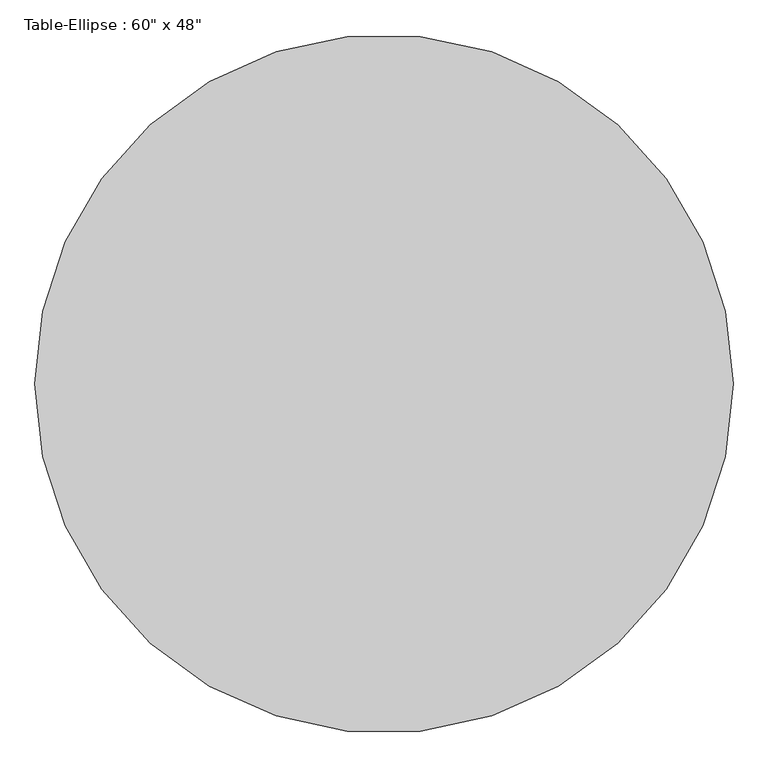
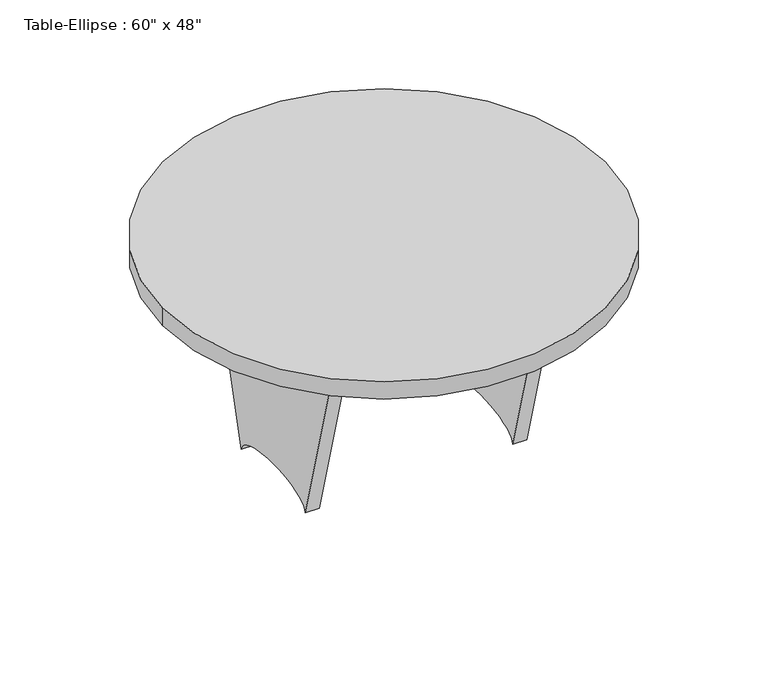
"""IFC4 building model written with IfcOpenShell, lengths in millimetres: furniture geometry."""

from ifc_helpers import new_model, si_unit, point, frame, origin, place, context, project, spatial, circle_curve, ellipse_curve, trimmed, source, transform, mapped, element, save
from ifc_brep_helpers import plane_surface, extruded_surface, advanced_brep


def furniture_c897acec(model_context):
    return source(origin(), model_context, "Body", "AdvancedBrep", [
        advanced_brep(
        [(-266.7, 19.05, 558.8), (266.7, 19.05, 558.8), (266.7, 19.05, 372.5333333), (-266.7, 19.05, 372.5333333), (-266.7, -19.05, 558.8), (-266.7, -19.05, 372.5333333), (266.7, -19.05, 372.5333333), (266.7, -19.05, 558.8)],
        [
            (0, 1),
            (1, 2),
            (2, 3, ellipse_curve(frame((0.0, 19.05, 372.5333333), z_axis=(0.0, -1.0, 0.0), x_axis=(1.0, 0.0, 0.0)), 266.7, 101.6)),
            (3, 0),
            (4, 5),
            (5, 6, ellipse_curve(frame((0.0, -19.05, 372.5333333), z_axis=(0.0, 1.0, 0.0), x_axis=(1.0, 0.0, 0.0)), 266.7, 101.6)),
            (6, 7),
            (7, 4),
            (0, 4),
            (7, 1),
            (6, 2),
            (5, 3),
        ],
        [
            plane_surface(frame((-266.7, 19.05, 558.8), z_axis=(0.0, 1.0, 0.0), x_axis=(1.0, 0.0, 0.0))),
            plane_surface(frame((-266.7, -19.05, 558.8), z_axis=(0.0, -1.0, 0.0), x_axis=(-1.0, 0.0, 0.0))),
            plane_surface(frame((-266.7, 19.05, 558.8), z_axis=(0.0, 0.0, 1.0), x_axis=(0.0, -1.0, 0.0))),
            plane_surface(frame((266.7, 19.05, 558.8), z_axis=(1.0, 0.0, 0.0), x_axis=(0.0, -1.0, 0.0))),
            extruded_surface(trimmed(ellipse_curve(frame((0.0, -57.15, 372.5333333), z_axis=(0.0, -1.0, 0.0), x_axis=(1.0, 0.0, 0.0)), 266.7, 101.6), [point((266.7, -57.15, 372.5333333))], [point((-266.7, -57.15, 372.5333333))], True, "CARTESIAN"), (0.0, 38.099999999999994, 0.0), 38.099999999999994),
            plane_surface(frame((-266.7, 19.05, 372.5333333), z_axis=(-1.0, 0.0, 0.0), x_axis=(0.0, -1.0, 0.0))),
        ],
        [
            (0, [[1, 2, 3, 4]]),
            (1, [[5, 6, 7, 8]]),
            (2, [[-1, 9, -8, 10]]),
            (3, [[-2, -10, -7, 11]]),
            (4, [[-3, -11, -6, 12]]),
            (5, [[-4, -12, -5, -9]]),
        ],
    ),
        advanced_brep(
        [(304.8, 304.8, 558.8), (304.8, -304.8, 558.8), (304.8, -152.4, 0.0), (304.8, 152.4, 0.0), (266.7, 304.8, 558.8), (266.7, 152.4, 0.0), (266.7, -152.4, 0.0), (266.7, -304.8, 558.8)],
        [
            (0, 1),
            (1, 2),
            (2, 3, ellipse_curve(frame((304.8, 0.0, 0.0), z_axis=(-1.0, 0.0, 0.0), x_axis=(0.0, 1.0, 0.0)), 152.4, 50.8)),
            (3, 0),
            (4, 5),
            (5, 6, ellipse_curve(frame((266.7, 0.0, 0.0), z_axis=(1.0, 0.0, 0.0), x_axis=(0.0, 1.0, 0.0)), 152.4, 50.8)),
            (6, 7),
            (7, 4),
            (0, 4),
            (7, 1),
            (6, 2),
            (5, 3),
        ],
        [
            plane_surface(frame((304.8, -304.8, 558.8), z_axis=(1.0, 0.0, 0.0), x_axis=(0.0, -1.0, 0.0))),
            plane_surface(frame((266.7, -304.8, 558.8), z_axis=(-1.0, 0.0, 0.0), x_axis=(0.0, 1.0, 0.0))),
            plane_surface(frame((304.8, 304.8, 558.8), z_axis=(0.0, 0.0, 1.0), x_axis=(-1.0, 0.0, 0.0))),
            plane_surface(frame((304.8, -304.8, 558.8), z_axis=(0.0, -0.9647638212377304, -0.2631174057921153), x_axis=(-1.0, 0.0, 0.0))),
            extruded_surface(trimmed(ellipse_curve(frame((228.6, 0.0, 0.0), z_axis=(-1.0, 0.0, 0.0), x_axis=(0.0, 1.0, 0.0)), 152.4, 50.8), [point((228.6, -152.4, 0.0))], [point((228.6, 152.4, 0.0))], True, "CARTESIAN"), (38.099999999999994, 0.0, 0.0), 38.099999999999994),
            plane_surface(frame((304.8, 152.4, 0.0), z_axis=(0.0, 0.9647638212377352, -0.2631174057920975), x_axis=(-1.0, 0.0, 0.0))),
        ],
        [
            (0, [[1, 2, 3, 4]]),
            (1, [[5, 6, 7, 8]]),
            (2, [[-1, 9, -8, 10]]),
            (3, [[-2, -10, -7, 11]]),
            (4, [[-3, -11, -6, 12]]),
            (5, [[-4, -12, -5, -9]]),
        ],
    ),
        advanced_brep(
        [(-266.7, 304.8, 558.8), (-266.7, -304.8, 558.8), (-266.7, -152.4, 0.0), (-266.7, 152.4, 0.0), (-304.8, 304.8, 558.8), (-304.8, 152.4, 0.0), (-304.8, -152.4, 0.0), (-304.8, -304.8, 558.8)],
        [
            (0, 1),
            (1, 2),
            (2, 3, ellipse_curve(frame((-266.7, 0.0, 0.0), z_axis=(-1.0, 0.0, 0.0), x_axis=(0.0, 1.0, 0.0)), 152.4, 50.8)),
            (3, 0),
            (4, 5),
            (5, 6, ellipse_curve(frame((-304.8, 0.0, 0.0), z_axis=(1.0, 0.0, 0.0), x_axis=(0.0, 1.0, 0.0)), 152.4, 50.8)),
            (6, 7),
            (7, 4),
            (0, 4),
            (7, 1),
            (6, 2),
            (5, 3),
        ],
        [
            plane_surface(frame((-266.7, -304.8, 558.8), z_axis=(1.0, 0.0, 0.0), x_axis=(0.0, -1.0, 0.0))),
            plane_surface(frame((-304.8, -304.8, 558.8), z_axis=(-1.0, 0.0, 0.0), x_axis=(0.0, 1.0, 0.0))),
            plane_surface(frame((-266.7, 304.8, 558.8), z_axis=(0.0, 0.0, 1.0), x_axis=(-1.0, 0.0, 0.0))),
            plane_surface(frame((-266.7, -304.8, 558.8), z_axis=(0.0, -0.9647638212377301, -0.26311740579211657), x_axis=(-1.0, 0.0, 0.0))),
            extruded_surface(trimmed(ellipse_curve(frame((-342.9, 0.0, 0.0), z_axis=(-1.0, 0.0, 0.0), x_axis=(0.0, 1.0, 0.0)), 152.4, 50.8), [point((-342.9, -152.4, 0.0))], [point((-342.9, 152.4, 0.0))], True, "CARTESIAN"), (38.099999999999966, 0.0, 0.0), 38.099999999999966),
            plane_surface(frame((-266.7, 152.4, 0.0), z_axis=(0.0, 0.9647638212377332, -0.2631174057921053), x_axis=(-1.0, 0.0, 0.0))),
        ],
        [
            (0, [[1, 2, 3, 4]]),
            (1, [[5, 6, 7, 8]]),
            (2, [[-1, 9, -8, 10]]),
            (3, [[-2, -10, -7, 11]]),
            (4, [[-3, -11, -6, 12]]),
            (5, [[-4, -12, -5, -9]]),
        ],
    ),
        advanced_brep(
        [(-609.6, 0.0, 609.6), (609.6, 0.0, 609.6), (-609.6, 0.0, 558.8), (609.6, 0.0, 558.8)],
        [
            (0, 1, circle_curve(frame((0.0, 0.0, 609.6), z_axis=(0.0, 0.0, 1.0), x_axis=(1.0, 0.0, 0.0)), 609.6)),
            (1, 0, circle_curve(frame((0.0, 0.0, 609.6), z_axis=(0.0, 0.0, 1.0), x_axis=(1.0, 0.0, 0.0)), 609.6)),
            (2, 3, ellipse_curve(frame((0.0, 0.0, 558.8), z_axis=(0.0, 0.0, -1.0), x_axis=(1.0, 0.0, 0.0)), 609.6, 609.6)),
            (3, 2, ellipse_curve(frame((0.0, 0.0, 558.8), z_axis=(0.0, 0.0, -1.0), x_axis=(1.0, 0.0, 0.0)), 609.6, 609.6)),
            (0, 2),
            (3, 1),
        ],
        [
            plane_surface(frame((609.6, 0.0, 609.6), z_axis=(0.0, 0.0, 1.0), x_axis=(0.0, 1.0, 0.0))),
            plane_surface(frame((609.6, 0.0, 558.8), z_axis=(0.0, 0.0, -1.0), x_axis=(0.0, -1.0, 0.0))),
            extruded_surface(trimmed(ellipse_curve(frame((0.0, 0.0, 508.0), z_axis=(0.0, 0.0, 1.0), x_axis=(1.0, 0.0, 0.0)), 609.6, 609.6), [point((-609.6, 0.0, 508.0))], [point((609.6, 0.0, 508.0))], True, "CARTESIAN"), (0.0, 0.0, 50.799999999999955), 50.799999999999955),
            extruded_surface(trimmed(ellipse_curve(frame((0.0, 0.0, 508.0), z_axis=(0.0, 0.0, 1.0), x_axis=(1.0, 0.0, 0.0)), 609.6, 609.6), [point((609.6, 0.0, 508.0))], [point((-609.6, 0.0, 508.0))], True, "CARTESIAN"), (0.0, 0.0, 50.799999999999955), 50.799999999999955),
        ],
        [
            (0, [[1, 2]]),
            (1, [[3, 4]]),
            (2, [[-1, 5, -4, 6]]),
            (3, [[-2, -6, -3, -5]]),
        ],
    ),
    ])


if __name__ == "__main__":
    model = new_model("IFC4")
    model_context = context("Model", 3, world=origin())
    ifc_project = project(units=[si_unit("LENGTHUNIT", "METRE", prefix="MILLI")], contexts=[model_context])
    site = spatial("IfcSite", under=ifc_project)
    building = spatial("IfcBuilding", under=site)
    placement = place(None, origin())
    furniture_shape = furniture_c897acec(model_context)
    element("IfcFurniture", 1, ObjectType="Table-Ellipse : 60\" x 48\"", at=placement, inside=building, context=model_context, shape_type="MappedRepresentation", body=[
        mapped(furniture_shape, transform((0.0, 0.0, 0.0), x_axis=(1.0, 0.0, 0.0), y_axis=(0.0, 1.0, 0.0), z_axis=(0.0, 0.0, 1.0))),
    ])
    save(model, "model.ifc")

# Revit data of these elements
# Type "Table-Ellipse : 60\" x 48\""
#   Assembly Code = "E2020200"
#   Half Width = 2' - 0"
#   Half Length = 2' - 0"
#   Height = 2' - 0"
#   Length = 4' - 0"
#   Width = 4' - 0"
#   Base Material = Birch
#   Top Material = Birch
#   Default Elevation = 0
# Element 1 (IfcFurniture, "Table-Ellipse : 60\" x 48\"")
#   Materials on its faces: "Birch"
# Materials
#   "Birch": class "Wood", colour RGB 224 178 126, transparency 0, Description = "Betula Alleghaniensis", Cost = 0
